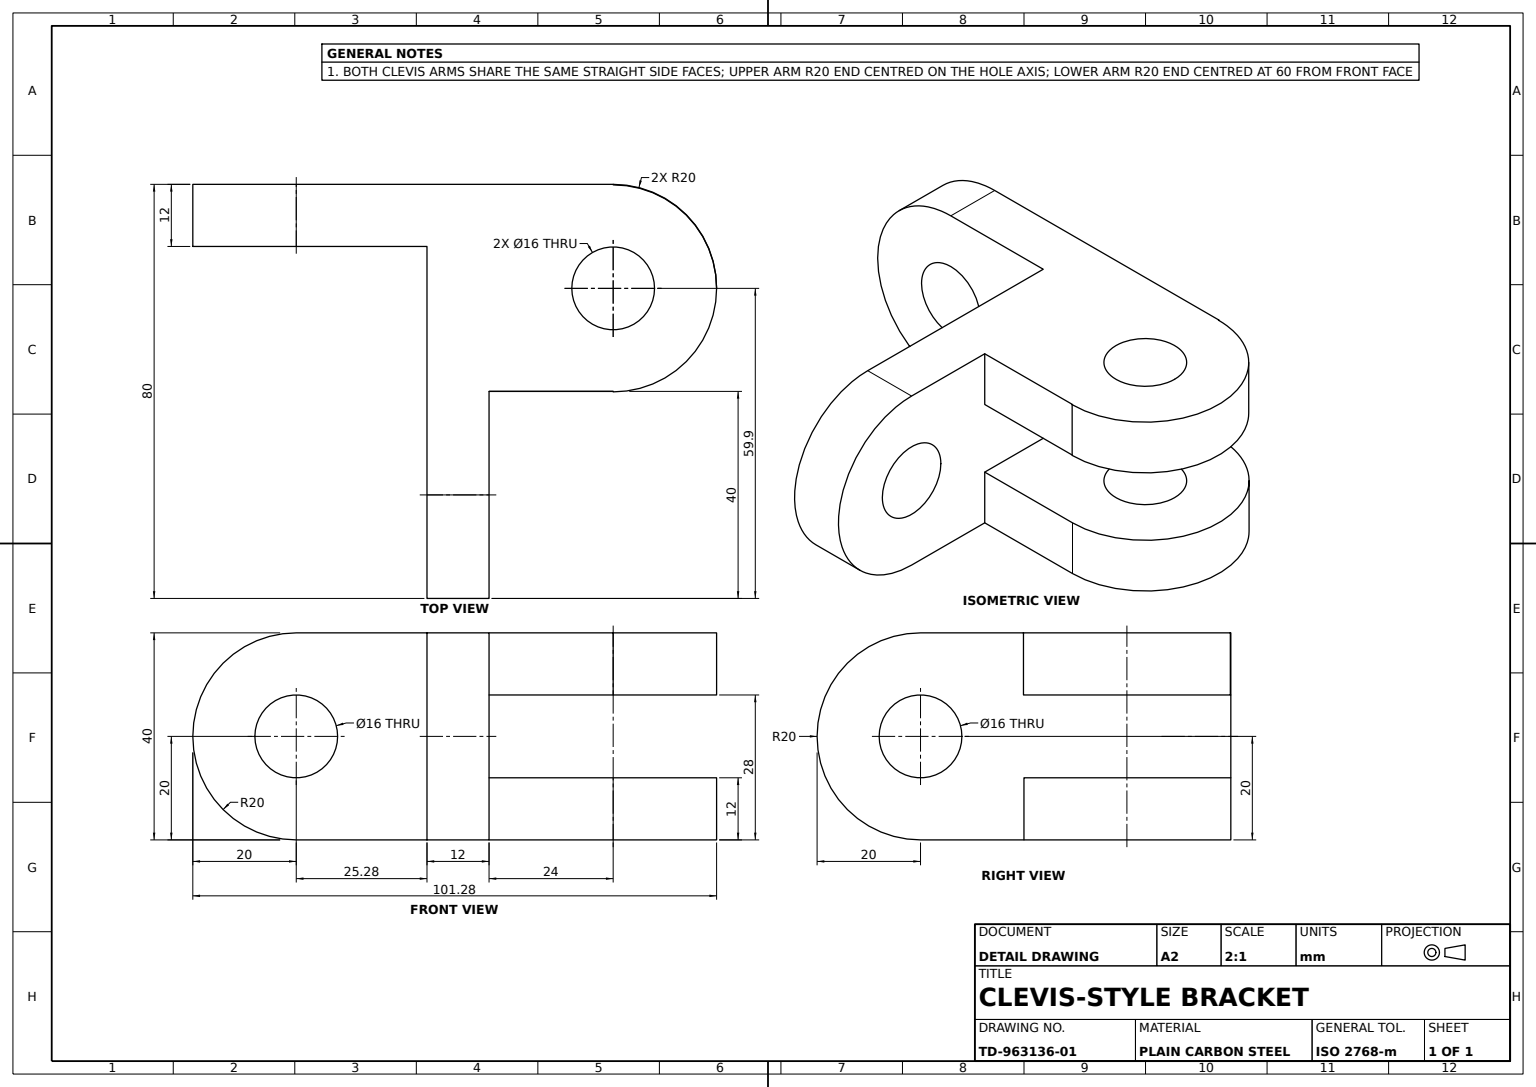
SolidWorks part; units mm, degrees
material "Plain Carbon Steel"
ref_plane "Front Plane" through (0, 0, 0) normal (0, 0, 1) x (1, 0, 0)
ref_plane "Top Plane" through (0, 0, 0) normal (0, 1, 0) x (1, 0, 0)
ref_plane "Right Plane" through (0, 0, 0) normal (1, 0, 0) x (0, 0, -1)
sketch "Base Profile Sketch" plane through (0, 0, 0) normal (0, 0, 1) x (1, 0, 0)
  line L0 (-33.1959, 0) -> (60, 0) construction
  line L1 (0, 0) -> (60, 0)
  line L4 (0, 0) -> (60, 0)
  line L5 (0, 0) -> (0, 40)
  line L6 (0, 40) -> (60, 40)
  arc A0 (60, 0) -> (60, 40) centre (60, 20) ccw
  dimension "D3" = 20
  dimension "D1" = 60
  dimension "D2" = 40
  dimension "D4" = 60
extrude "Base Bracket" add sketch "Base Profile Sketch" along normal mid plane 12 contours L1 A0 L6 L5
sketch "Upper Lug Plate Sketch" plane through (0, 40, 0) normal (0, 1, 0) x (1, 0, 0)
  line L1 (0, 6) -> (40, 6)
  line L2 (0, 6) -> (0, 30)
  line L4 (40, 6) -> (40, 30)
  arc A0 (40, 30) -> (0, 30) centre (20, 30) ccw
  dimension "D2" = 40
  dimension "D1" = 24
extrude "Upper Lug Plate" add sketch "Upper Lug Plate Sketch" against normal blind 12 from offset 28 contours L2 A0 L4 L1 offset against normal yes
sketch "Upper Lug End Sketch" plane through (0, 40, 0) normal (0, 1, 0) x (1, 0, 0)
  line L0 (40.0953, 30) -> (40, 30)
  line L1 (0, 6) -> (40, 6)
  line L2 (0, 6) -> (0, 30)
  line L3 (0, 30) -> (0.0953, 30)
  line L4 (40, 6) -> (40, 30)
  arc A0 (40.0953, 30) -> (0.0953, 30) centre (20.0953, 30) ccw
  dimension "D2" = 20
  dimension "D1" = 24
  dimension "D3" = 30
  dimension "D4" = 20.0953
  dimension "D5" = 0.0953
extrude "Upper Lug Rounded End" add sketch "Upper Lug End Sketch" against normal blind 12
sketch "Upper Lug Hole Sketch" plane through (0, 40, 0) normal (0, 1, 0) x (1, 0, 0)
  circle A0 centre (20.0953, 30) radius 8
  dimension "D1" = 16
extrude "Upper Lug Hole Ø16" cut sketch "Upper Lug Hole Sketch" against normal through all
sketch "Side Lug Sketch" plane through (0, 0, 0) normal (-1, 0, 0) x (0, 0, 1)
  line L0 (6, 0) -> (-30, 0) construction
  line L1 (6, 40) -> (31.2796, 40)
  line L2 (6, 40) -> (6, 0)
  line L3 (6, 0) -> (31.2796, 0)
  arc A0 (31.2796, 0) -> (31.2796, 40) centre (31.2796, 20) ccw
  dimension "D1" = 25.2796
extrude "Side Lug" add sketch "Side Lug Sketch" against normal blind 12
sketch "Side Lug Hole Sketch" plane through (12, 0, 0) normal (1, 0, 0) x (0, 0, -1)
  circle A0 centre (-31.2796, 20) radius 8
  dimension "D1" = 16
extrude "Side Lug Hole Ø16" cut sketch "Side Lug Hole Sketch" against normal through all
sketch "Base Hole Sketch" plane through (0, 0, 6) normal (0, 0, 1) x (1, 0, 0)
  circle A0 centre (60, 20) radius 8
  dimension "D1" = 16
extrude "Base Hole Ø16" cut sketch "Base Hole Sketch" against normal through all
